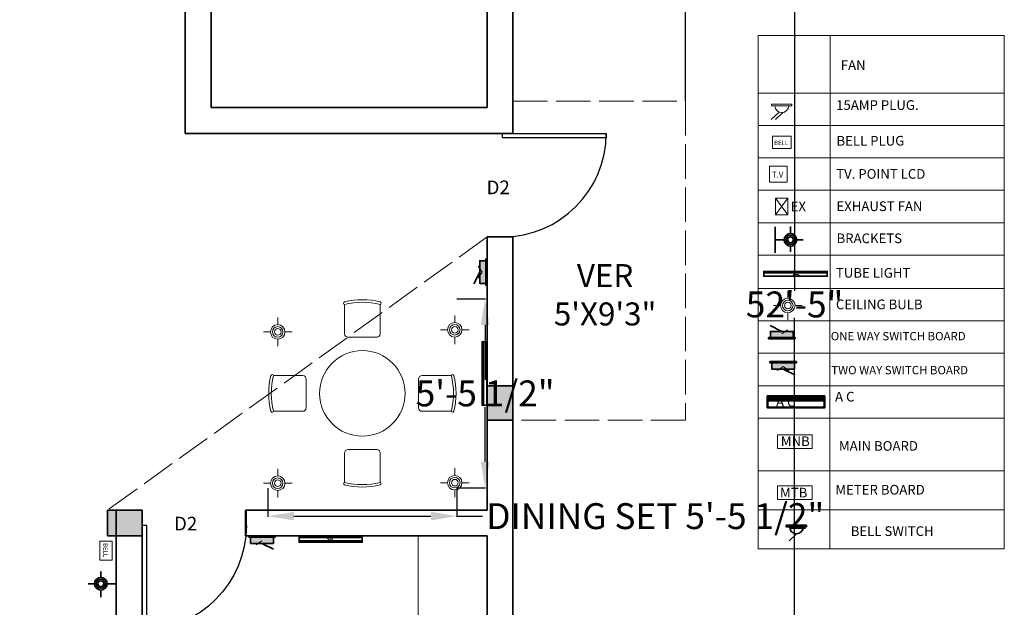
# Model space of a CAD drawing. Units: inches. Extents: x 68 to 1275, y 90 to 1276.
# Tile 5 of 6: x 916 to 1259, y 813 to 1017. Entities that reach past the tile are written whole.
import ezdxf

# ---------------------------------------------------------------- set-up
doc = ezdxf.new("R2010")
doc.units = ezdxf.units.IN
doc.header["$MEASUREMENT"] = 0
doc.linetypes.add('ACAD_ISO02W100', pattern=[15, 12, -3])
for name, color, linetype, lineweight in [('A -Elec', 6, 'Continuous', 18), ('A-ANNO-TEXT', 7, 'Continuous', 18), ('A-AREA-IDEN', 7, 'Continuous', 18), ('A-FLOR-FIXT', 9, 'Continuous', 18), ('A-FLOR-OVHD', 8, 'ACAD_ISO02W100', 13), ('A-WALL', 7, 'Continuous', 35), ('COLUMN', 150, 'Continuous', 35), ('DIM', 2, 'Continuous', 18), ('DOOR', 15, 'Continuous', 25), ('E-ANNO-LEGD', 8, 'Continuous', 13), ('E-ANNO-TEXT', 7, 'Continuous', 18), ('E-EQPM', 1, 'Continuous', 18), ('E-LITE', 6, 'Continuous', 18), ('E-POWR', 1, 'Continuous', 18), ('E-REFR', 8, 'ACAD_ISO02W100', 13), ('Elec', 1, 'Continuous', 35), ('FURN', 163, 'Continuous', 18)]:
    doc.layers.add(name, color=color, linetype=linetype, lineweight=lineweight)
doc.styles.get("Standard").update_dxf_attribs({"font": 'arial.ttf'})
doc.dimstyles.get("Standard").update_dxf_attribs({"dimtxt": 9, "dimasz": 9, "dimexe": 0.18, "dimexo": 0.0625, "dimgap": 0.09, "dimtad": 0, "dimtih": 1, "dimtoh": 1, "dimdec": 1, "dimzin": 0, "dimdsep": 46, "dimlunit": 3, "dimtxsty": 'Standard', "dimcen": 0.09, "dimadec": 0, "dimazin": 0, "dimtfac": 1, "dimtdec": 1, "dimtofl": 0, "dimtmove": 0, "dimatfit": 3, "dimfxl": 1, "dimtolj": 1, "dimtzin": 0, "dimarcsym": 0})

# ---------------------------------------------------------------- blocks, each defined once
blk = doc.blocks.new('*U2')
for p, q in [((0, 0), (-1e-16, -5.999999999999999)), ((40, -6e-16), (40, -6))]:
    blk.add_line(p, q)
blk.add_lwpolyline([(0, 0), (5.6e-15, 40), (1.750000000000007, 40), (1.749999999999998, -7e-16)], close=True)
blk.add_arc((0, 0), 40, 0, 90)
blk = doc.blocks.new('C')
h = blk.add_hatch(color=256)
h.dxf.hatch_style = 1
h.paths.add_polyline_path([(745.8101109123093, 845.9819968167334), (745.8101109123093, 857.9819968167335), (736.8101109123093, 857.9819968167335), (736.8101109123093, 845.9819968167334)])
for p, q in [((745.8101109123093, 857.9819968167335), (736.8101109123093, 857.9819968167335)), ((736.8101109123093, 857.9819968167335), (736.8101109123093, 845.9819968167334)), ((745.8101109123093, 845.9819968167334), (745.8101109123093, 857.9819968167335)), ((736.8101109123093, 845.9819968167334), (745.8101109123093, 845.9819968167334))]:
    blk.add_line(p, q)
blk = doc.blocks.new('DCHARRND')
for p, q in [((-10, -2.638149999995254), (-10, -18.99994999999526)), ((10, -18.99994999999526), (10, -2.638149999995254)), ((-8, -20.99994999999526), (8, -20.99994999999526))]:
    blk.add_line(p, q)
for centre, radius, start, end in [((0, -41.27199999999525), 41.27199999999525, 75.97797000000331, 104.0219999999933), ((-9.769699999999943, -1.946949999995245), 0.7532336000029903, 107.8004999997948, 188.6619999997561), ((-9.86489999999992, -2.000049999995248), 0.6522302000032755, 185.3118999999788, 258.0499999996009), ((0, -42.68031999999524), 41.27199999999525, 75.97797000000331, 104.0219999999933), ((9.769700000000057, -1.946949999995245), 0.7532335999955265, 351.3380000002426, 72.19952999994322), ((9.865000000000009, -2.000049999995248), 0.6522301999967041, 281.9500000003992, 354.6881000000212), ((-8, -18.99994999999526), 2, 180, 270), ((8, -18.99994999999526), 2, 270, 0)]:
    blk.add_arc(centre, radius, start, end)
blk = doc.blocks.new('*U23')
at = {"layer": 'FURN', "xscale": -0.8325683909312864, "yscale": 0.8325683909312864, "zscale": 0.8325683909312864, "rotation": 270}
blk.add_blockref('DCHARRND', (8.741947290566713, 3.1832e-12), dxfattribs=at)
blk = doc.blocks.new('*U24')
at = {"color": 0, "linetype": 'ByBlock', "lineweight": -2, "transparency": 16777216}
for p, rotation in [((1883.427219751119, 1330.162309104793), 90.00000000000006), ((1848.567433110135, 1295.302522463815), 180), ((1883.427219751113, 1260.442735822831), 270.0000000000001)]:
    blk.add_blockref('*U23', p, dxfattribs=dict(at, rotation=rotation))
blk.add_blockref('*U23', (1918.287006392097, 1295.302522463809), dxfattribs=at)
blk = doc.blocks.new('DIN')
blk.add_circle((1883.427219751116, 1295.302522463812), 19.90213577479114)
blk.add_blockref('*U24', (0, 0))
blk = doc.blocks.new('BELL SWITCH')
at = {"layer": 'Elec'}
for p, q in [((4981.810695824261, 3401.308516663301), (4981.810695824261, 3402.267205949833)), ((4981.810695824261, 3402.267205949833), (4993.567325880143, 3402.267205949833)), ((4993.567325880143, 3401.308516663301), (4981.810695824261, 3401.308516663301)), ((4993.567325880143, 3402.267205949833), (4993.567325880143, 3401.308516663301)), ((4987.689010852202, 3397.361748155474), (4983.521874140887, 3393.30038126191))]:
    blk.add_line(p, q, dxfattribs=at)
blk.add_arc((4987.689010852202, 3401.308516663301), 3.946768507828181, 180, 0, dxfattribs=at)
blk = doc.blocks.new('splight')
at = {"layer": 'Elec'}
for p, q in [((4618.165493646445, 527.1595508907546), (4627.57380882646, 527.1595508907546)), ((4622.869651236451, 527.1595508907546), (4622.869651236451, 523.8688723625129)), ((4620.576181531769, 521.5754026578305), (4618.052205676129, 521.5754026578305)), ((4625.163120941137, 521.5754026578305), (4627.232633020232, 521.5754026578305)), ((4622.869651236451, 519.2819329531479), (4622.869651236451, 517.0346704452847))]:
    blk.add_line(p, q, dxfattribs=at)
for radius in [2.293469704682637, 1.668469704682639, 1.043469704682639]:
    blk.add_circle((4622.869651236451, 521.5754026578305), radius, dxfattribs=at)
blk = doc.blocks.new('CIELING')
at = {"layer": 'A -Elec'}
for p, q in [((1070.869500591183, -8395.655580837194), (1070.869500591183, -8391.485789029257)), ((1066.613971407157, -8399.911110021205), (1062.44417959922, -8399.911110021205)), ((1075.125029775208, -8399.911110021205), (1079.294821583145, -8399.911110021205)), ((1070.869500591183, -8408.33643101315), (1070.869500591183, -8404.166639205214))]:
    blk.add_line(p, q, dxfattribs=at)
for radius in [4.255529184009533, 3.095842734009534, 1.936156284009533]:
    blk.add_circle((1070.869500591183, -8399.911110021205), radius, dxfattribs=at)
blk = doc.blocks.new('tube')
at = {"layer": 'A -Elec'}
for p, q in [((4592.607752765609, 556.7543292074987), (4641.607752765609, 556.7543292074987)), ((4592.607752765609, 555.2543292074988), (4592.607752765609, 556.7543292074987)), ((4592.607752765609, 552.7543292074987), (4592.607752765609, 555.2543292074988)), ((4592.607752765609, 552.7543292074987), (4641.607752765609, 552.7543292074987)), ((4593.107752765609, 555.2543292074988), (4593.107752765609, 556.7543292074987)), ((4593.107752765609, 556.3299144522243), (4593.407752765609, 556.3299144522243)), ((4593.107752765609, 556.2104979518087), (4593.407752765609, 556.2104979518087)), ((4593.107752765609, 555.8060867251079), (4593.407752765609, 555.8060867251079)), ((4593.107752765609, 555.6866702246923), (4593.407752765609, 555.6866702246923)), ((4641.107752765608, 555.2543292074988), (4593.107752765609, 555.2543292074988)), ((4593.107752765609, 555.2543292074988), (4593.107752765609, 553.2543292074988)), ((4593.107752765609, 553.2543292074988), (4593.107752765609, 555.2543292074988)), ((4593.107752765609, 553.2543292074988), (4641.607752765609, 553.2543292074988)), ((4593.407752765609, 555.2543292074988), (4593.407752765609, 556.7543292074987)), ((4593.407752765609, 556.5043292074988), (4640.807752765609, 556.5043292074988)), ((4593.407752765609, 556.2543292074987), (4640.807752765609, 556.2543292074987)), ((4593.407752765609, 556.0043292074988), (4640.807752765609, 556.0043292074988)), ((4593.407752765609, 555.7543292074988), (4640.807752765609, 555.7543292074988)), ((4593.407752765609, 555.5043292074988), (4640.807752765609, 555.5043292074988)), ((4640.807752765609, 555.2543292074988), (4640.807752765609, 556.7543292074987)), ((4640.807752765609, 556.3299144522243), (4641.107752765608, 556.3299144522243)), ((4640.807752765609, 556.2104979518087), (4641.107752765608, 556.2104979518087)), ((4640.807752765609, 555.8060867251079), (4641.107752765608, 555.8060867251079)), ((4640.807752765609, 555.6866702246923), (4641.107752765608, 555.6866702246923)), ((4641.107752765608, 556.7543292074987), (4641.107752765608, 555.2543292074988)), ((4641.107752765608, 555.2543292074988), (4641.107752765608, 556.7543292074987)), ((4641.107752765608, 553.2543292074988), (4641.107752765608, 555.2543292074988)), ((4641.607752765609, 556.7543292074987), (4641.607752765609, 555.2543292074988)), ((4641.607752765609, 552.7543292074987), (4641.607752765609, 555.2543292074988))]:
    blk.add_line(p, q, dxfattribs=at)
for points in [[(4615.603450108063, 553.2543292074988), (4619.112055423154, 553.2543292074988), (4619.112055423154, 554.3062122222327), (4615.603450108063, 554.3062122222327)], [(4619.112055423154, 553.7802707148657), (4619.112055423154, 553.7802707148657), (4619.112055423154, 553.7802707148657), (4619.112055423154, 553.7802707148657)], [(4619.112055423154, 553.7802707148657), (4619.813791770798, 553.7802707148657), (4619.813791770798, 553.2543292074988), (4619.112055423154, 553.2543292074988)]]:
    blk.add_lwpolyline(points, close=True, dxfattribs=at)
blk = doc.blocks.new('ac')
at = {"layer": 'Elec'}
for p, q in [((12718.33512872629, -53.78451556294852), (12674.35721837807, -53.78451556294852)), ((12674.35721837806, -63.01930683579224), (12674.35721837807, -53.78451556294852)), ((12674.88506837807, -57.52248662285011), (12717.80727872628, -57.52248662285011)), ((12675.81311487755, -57.52248662285011), (12675.81311487755, -53.78451556294851)), ((12717.02869991749, -54.85019267976269), (12675.81311487755, -54.85019267976269)), ((12717.02869991749, -56.20859049643797), (12675.81311487755, -56.20859049643797)), ((12717.02869991748, -57.52248662285011), (12717.02869991749, -53.78451556294851)), ((12718.33512872629, -63.01930683579224), (12718.33512872629, -53.78451556294852)), ((12718.33512872629, -63.01930683579224), (12674.35721837806, -63.01930683579224))]:
    blk.add_line(p, q, dxfattribs=at)
at = {"layer": 'Elec', "ltscale": 0.1}
for p, q in [((12674.88506837807, -61.49145683579366), (12674.88506837807, -53.78451556294851)), ((12717.02869991749, -54.35872395628861), (12675.81311487755, -54.35872395628861)), ((12717.02869991749, -55.65507023101156), (12675.81311487755, -55.65507023101157)), ((12717.02869991749, -56.84485043173038), (12675.81311487755, -56.84485043173037)), ((12717.80727872628, -61.49145683579366), (12717.80727872628, -53.78451556294851)), ((12716.80727872628, -62.49145683579365), (12675.88506837807, -62.49145683579365))]:
    blk.add_line(p, q, dxfattribs=at)
at = {"layer": 'Elec'}
for centre, start, end in [((12675.88506837807, -61.49145683579366), 180, 270), ((12716.80727872628, -61.49145683579366), 270, 0)]:
    blk.add_arc(centre, 1, start, end, dxfattribs=at)
blk = doc.blocks.new('elec box')
at = {"layer": 'Elec'}
blk.add_hatch(color=256, dxfattribs=at).paths.add_polyline_path([(3828.234962737587, 599.2881263179643), (3828.234962737587, 594.7881263179643), (3844.734962737589, 594.7881263179643), (3844.734962737589, 599.2881263179643)])
for p, q in [((3836.484962737588, 599.2881263179643), (3828.066979685118, 603.4529863194257)), ((3846.10280273742, 594.7881263179643), (3826.830962060027, 594.7881263179643)), ((3826.830962060027, 594.7881263179643), (3826.830962060027, 593.8893551118417)), ((3826.830962060027, 593.8893551118417), (3846.10280273742, 593.8893551118417)), ((3846.10280273742, 593.8893551118417), (3846.10280273742, 594.7881263179643))]:
    blk.add_line(p, q, dxfattribs=at)
blk.add_lwpolyline([(3828.234962737587, 594.7881263179643), (3828.234962737587, 599.2881263179643), (3844.734962737589, 599.2881263179643), (3844.734962737589, 594.7881263179643), (3828.234962737587, 594.7881263179643)], dxfattribs=at)
blk = doc.blocks.new('SWITCHBOARD-ONE-WAY')
blk.add_line((4.634474659967281, 1.72886330620372), (6.643170124125163, 3.124132868275296))
at = {"xscale": 0.480395109260985, "yscale": 0.480395109260985, "zscale": 0.480395109260985}
blk.add_blockref('elec box', (-1838.391242964724, -285.3017071861163), dxfattribs=at)
blk = doc.blocks.new('SWITCHBOARD-TWO-WAY')
for p, q in [((4.623595448308151, 2.865329432813496), (2.614899984150042, 1.47005987070861)), ((4.623595442911664, 2.865329432846692), (6.622900514750199, 1.456637185270096))]:
    blk.add_line(p, q)
at = {"xscale": 0.480395109260985, "yscale": 0.480395109260985, "zscale": 0.480395109260985, "rotation": 180}
blk.add_blockref('elec box', (1847.649313070309, 289.8958999251334), dxfattribs=at)
blk = doc.blocks.new('BELL-POINT')
blk.add_lwpolyline([(1.95874658857e-05, 4.272243527406885), (6.55734876643055, 4.272243527406885), (6.55734876643055, -0.0002228979699339), (1.95874658857e-05, -0.0002228979699339)], close=True)
at = {"insert": (0.6440248614437678, 2.798299889551913), "char_height": 1.537264349632867, "attachment_point": 1}
blk.add_mtext('BELL', dxfattribs=at)
blk = doc.blocks.new('TV-POINT')
blk.add_lwpolyline([(2.2128117507e-06, 5.568118865895371), (6.100736396045249, 5.568118865895371), (6.100736396045249, -7.01044664311e-05), (2.2128117507e-06, -7.01044664311e-05)], close=True)
at = {"transparency": 33554676}
blk.add_lwpolyline([(2.2128117507e-06, 5.568118865895371), (6.100736396045249, 5.568118865895371), (6.100736396045249, -7.01044664311e-05), (2.2128117507e-06, -7.01044664311e-05)], close=True, dxfattribs=at)
at = {"insert": (0.8393167226115565, 3.647168321161302), "char_height": 2.003474701485161, "attachment_point": 1}
blk.add_mtext('T.V ', dxfattribs=at)
at = {"transparency": 33554676, "insert": (0.8393167226115565, 3.647168321161302), "char_height": 2.003474701485161, "attachment_point": 1}
blk.add_mtext('T.V ', dxfattribs=at)
blk = doc.blocks.new('MAIN-BOARD')
blk.add_lwpolyline([(0.0004361200251424, 4.703133274055858), (12.06279134155943, 4.703133274055858), (12.06279134155943, 0.0003298403245253), (0.0004361200251424, 0.0003298403245253)], close=True)
blk.add_text('MNB', height=3.362765764821897).set_placement((1.14402048200327, 0.7969751531460361))
blk = doc.blocks.new('METER-BOARD')
blk.add_lwpolyline([(0.0004361200251424, 4.702354804303354), (12.06279134155943, 4.702354804303354), (12.06279134155943, -0.0004486294279786), (0.0004361200251424, -0.0004486294279786)], close=True)
blk.add_text('MTB', height=3.362765764821897).set_placement((0.8731259797250459, 0.6934873088445102))
blk = doc.blocks.new('*D65')
at = {"layer": 'Defpoints', "color": 0, "transparency": 16777216}
for p in [(1002.392096138563, 854.1861430656332), (1068.072978243499, 854.1861430656332), (1068.072978243499, 844.3340107498929)]:
    blk.add_point(p, dxfattribs=at)
at = {"layer": 'DIM', "color": 0, "lineweight": -2, "transparency": 16777216}
for p, q in [((1002.392096138563, 854.1236430656332), (1002.392096138563, 844.1540107498928)), ((1068.072978243499, 854.1236430656332), (1068.072978243499, 844.1540107498928)), ((1011.392096138563, 844.3340107498929), (1059.072978243499, 844.3340107498929)), ((1068.072978243499, 844.3340107498929), (1077.072978243499, 844.3340107498929))]:
    blk.add_line(p, q, dxfattribs=at)
at = {"layer": 'DIM', "color": 0, "transparency": 16777216}
for points in [[(1011.392096138563, 845.8340107498926), (1011.392096138563, 842.8340107498927), (1002.392096138563, 844.3340107498929)], [(1059.072978243499, 845.8340107498926), (1059.072978243499, 842.8340107498927), (1068.072978243499, 844.3340107498929)]]:
    blk.add_solid(points, dxfattribs=at)
at = {"layer": 'DIM', "color": 0, "transparency": 16777216, "insert": (1137.108749048411, 844.3340107498929), "char_height": 9, "attachment_point": 5}
blk.add_mtext('\\A1;DINING SET 5\'-5 1/2"', dxfattribs=at)
blk = doc.blocks.new('*D66')
at = {"layer": 'Defpoints', "color": 0, "transparency": 16777216}
for p in [(1068.0729782435, 919.8670251705701), (1077.92511055924, 919.8670251705701), (1068.0729782435, 854.1861430656338)]:
    blk.add_point(p, dxfattribs=at)
at = {"layer": 'DIM', "color": 0, "lineweight": -2, "transparency": 16777216}
for p, q in [((1068.1354782435, 919.8670251705701), (1078.10511055924, 919.8670251705701)), ((1077.92511055924, 910.8670251705701), (1077.92511055924, 891.7700629721265)), ((1077.92511055924, 863.1861430656337), (1077.92511055924, 882.2831052640774)), ((1068.1354782435, 854.1861430656338), (1078.10511055924, 854.1861430656338))]:
    blk.add_line(p, q, dxfattribs=at)
at = {"layer": 'DIM', "color": 0, "transparency": 16777216}
for points in [[(1076.425110559241, 910.8670251705701), (1079.42511055924, 910.8670251705701), (1077.92511055924, 919.8670251705701)], [(1076.425110559241, 863.1861430656337), (1079.42511055924, 863.1861430656337), (1077.92511055924, 854.1861430656338)]]:
    blk.add_solid(points, dxfattribs=at)
at = {"layer": 'DIM', "color": 0, "transparency": 16777216, "insert": (1077.92511055924, 887.0265841181014), "char_height": 9, "attachment_point": 5}
blk.add_mtext('\\A1;5\'-5 1/2"', dxfattribs=at)
blk = doc.blocks.new('*D112')
at = {"layer": 'Defpoints', "color": 0, "transparency": 16777216}
for p in [(1147.626284, 1270.418609), (718.626284, 1232.468609), (1147.626284, 988.6789849999999)]:
    blk.add_point(p, dxfattribs=at)
at = {"layer": 'DIM', "color": 0, "lineweight": -2, "transparency": 16777216}
for p, q in [((718.626284, 1232.531109), (718.626284, 1270.598609)), ((727.626284, 1270.418609), (917.5809633997271, 1270.418609)), ((1138.626284, 1270.418609), (948.6716046002728, 1270.418609)), ((1147.626284, 988.741485), (1147.626284, 1270.598609))]:
    blk.add_line(p, q, dxfattribs=at)
at = {"layer": 'DIM', "color": 0, "transparency": 16777216}
for points in [[(727.626284, 1271.918609), (727.626284, 1268.918609), (718.626284, 1270.418609)], [(1138.626284, 1271.918609), (1138.626284, 1268.918609), (1147.626284, 1270.418609)]]:
    blk.add_solid(points, dxfattribs=at)
at = {"layer": 'DIM', "color": 0, "transparency": 16777216, "insert": (933.1262839999999, 1270.418609), "char_height": 9, "attachment_point": 5}
blk.add_mtext('\\A1;35\'-9"', dxfattribs=at)
blk = doc.blocks.new('*D113')
at = {"layer": 'Defpoints', "color": 0, "transparency": 16777216}
for p in [(1087.626284, 1232.468609), (1185.576284000001, 1232.468609), (1087.626284, 603.4686090000002)]:
    blk.add_point(p, dxfattribs=at)
at = {"layer": 'DIM', "color": 0, "lineweight": -2, "transparency": 16777216}
for p, q in [((1087.688784, 1232.468609), (1185.756284000001, 1232.468609)), ((1185.576284000001, 1223.468609), (1185.576284000001, 922.6537658894956)), ((1185.576284000001, 612.4686090000002), (1185.576284000001, 913.2834521105051)), ((1087.688784, 603.4686090000002), (1185.756284000001, 603.4686090000002))]:
    blk.add_line(p, q, dxfattribs=at)
at = {"layer": 'DIM', "color": 0, "transparency": 16777216}
for points in [[(1184.076284000001, 1223.468609), (1187.076284000001, 1223.468609), (1185.576284000001, 1232.468609)], [(1184.076284000001, 612.4686090000002), (1187.076284000001, 612.4686090000002), (1185.576284000001, 603.4686090000002)]]:
    blk.add_solid(points, dxfattribs=at)
at = {"layer": 'DIM', "color": 0, "transparency": 16777216, "insert": (1185.576284000001, 917.9686089999998), "char_height": 9, "attachment_point": 5}
blk.add_mtext('\\A1;52\'-5"', dxfattribs=at)

msp = doc.modelspace()

# ---------------------------------------------------------------- linework, layer by layer
at = {"layer": 'A-FLOR-FIXT'}
msp.add_line((1054.626283693841, 837.4686089321809), (1054.626283693841, 729.4686089321808), dxfattribs=at)
at = {"layer": 'A-FLOR-OVHD'}
for p, q in [((1087.626283693841, 988.6789849601155), (1147.626283693841, 988.6789849601155)), ((1147.626283693841, 988.6789849601155), (1147.626283693841, 877.6789849601154)), ((1147.626283693841, 877.6789849601154), (1087.626283693841, 877.6789849601154))]:
    msp.add_line(p, q, dxfattribs=at)
at = {"layer": 'A-WALL'}
for p, q in [((1087.626283693841, 1232.468608932181), (1087.626283693841, 977.4686089321807)), ((973.626283693841, 1082.468608932181), (973.626283693841, 977.4686089321807)), ((982.626283693841, 1082.468608932181), (982.626283693841, 986.4686089321807)), ((1078.626283693841, 1082.468608932181), (1078.626283693841, 986.4686089321807)), ((982.626283693841, 986.4686089321807), (1078.626283693841, 986.4686089321807)), ((973.626283693841, 977.4686089321807), (1078.626283693841, 977.4686089321807)), ((1078.626283693841, 977.4686089321807), (1087.626283693841, 977.4686089321807)), ((1078.626283693841, 941.4686089321808), (1078.626283693841, 846.4686089321808)), ((1078.626283693841, 941.4686089321808), (1087.626283693841, 941.4686089321808)), ((1087.626283693841, 941.4686089321808), (1087.626283693841, 696.4686089321808)), ((949.6262836938411, 846.4686089321808), (958.6262836938411, 846.4686089321808)), ((949.6262836938411, 846.4686089321808), (949.6262836938411, 705.4686089321807)), ((958.6262836938411, 837.4686089321809), (958.6262836938411, 846.4686089321808)), ((994.626283693841, 846.4686089321808), (1078.626283693841, 846.4686089321808)), ((994.626283693841, 837.4686089321809), (994.626283693841, 846.4686089321808)), ((949.6262836938411, 837.4686089321809), (958.6262836938411, 837.4686089321809)), ((958.6262836938411, 837.4686089321809), (958.6262836938411, 705.4686089321807)), ((994.626283693841, 837.4686089321809), (1078.626283693841, 837.4686089321809)), ((1078.626283693841, 837.4686089321809), (1078.626283693841, 705.4686089321807))]:
    msp.add_line(p, q, dxfattribs=at)
at = {"layer": 'E-ANNO-LEGD'}
for p, q in [((1172.946309647792, 832.969593099326), (1172.946309647792, 1011.519571694431)), ((1258.530314853673, 1011.519571694431), (1172.946309647792, 1011.519571694431)), ((1197.924334482565, 1011.519571694431), (1197.781428473779, 832.969593099326)), ((1258.530314853665, 832.969593099326), (1258.530314853665, 1011.519571694431)), ((1258.530314853673, 991.4346260608072), (1172.946309647792, 991.4346260608072)), ((1258.530314853673, 991.4346260608239), (1172.946309647792, 991.4346260608239)), ((1258.530314853673, 980.1762997075286), (1172.946309647792, 980.1762997075286)), ((1258.530314853665, 968.9179733542502), (1172.946309647775, 968.9179733542502)), ((1258.530314853673, 957.6596470009549), (1172.946309647792, 957.6596470009549)), ((1258.530314853673, 946.4013206476765), (1172.946309647792, 946.4013206476765)), ((1258.530314853673, 935.142994294398), (1172.946309647792, 935.142994294398)), ((1258.530314853665, 923.4772036206607), (1172.946309647775, 923.4772036206607)), ((1258.530314853665, 912.2188772673657), (1172.946309647775, 912.2188772673657)), ((1258.530314853665, 900.960550914087), (1172.946309647775, 900.960550914087)), ((1258.530314853673, 889.702224560792), (1172.946309647792, 889.702224560792)), ((1258.530314853673, 878.4438982075135), (1172.946309647792, 878.4438982075135)), ((1258.530314853673, 860.0415084382558), (1172.946309647792, 860.0415084382558)), ((1258.530314853673, 846.505550768799), (1172.946309647792, 846.505550768799)), ((1258.530314853673, 832.9695930993256), (1172.946309647792, 832.9695930993256))]:
    msp.add_line(p, q, dxfattribs=at)
at = {"layer": 'E-EQPM'}
for p, q in [((1178.958906185277, 954.9375739626636), (1183.282462168619, 949.1728326515301)), ((1183.282462168619, 954.9375739626636), (1178.958906185277, 949.1728326515301))]:
    msp.add_line(p, q, dxfattribs=at)
msp.add_lwpolyline([(1183.282462168619, 954.9375739626636), (1178.958906185277, 954.9375739626636), (1178.958906185277, 949.1728326515301), (1183.282462168619, 949.1728326515301)], close=True, dxfattribs=at)
at = {"layer": 'E-POWR'}
for p, q in [((1177.590791939301, 987.6368285849791), (1184.650576414587, 987.6368285849791)), ((1177.590791939301, 987.06114152929), (1177.590791939301, 987.6368285849791)), ((1184.650576414587, 987.06114152929), (1177.590791939301, 987.06114152929)), ((1184.650576414587, 987.6368285849791), (1184.650576414587, 987.06114152929)), ((1180.178658963754, 984.8863915189612), (1177.475973345754, 982.2523051778636)), ((1181.47769277534, 984.6911311686061), (1178.975352655661, 982.2523051778636))]:
    msp.add_line(p, q, dxfattribs=at)
msp.add_arc((1181.120684176957, 987.06114152929), 2.370010360678894, 180, 0, dxfattribs=at)
at = {"layer": 'E-REFR'}
msp.add_line((1078.626283693841, 941.4425014682521), (946.626283693841, 846.4686089321808), dxfattribs=at)

# ---------------------------------------------------------------- block references
at = {"layer": 'COLUMN'}
msp.add_blockref('C', (341.8161727815318, 31.69698814338199), dxfattribs=at)
at = {"layer": 'COLUMN', "rotation": 270}
msp.add_blockref('C', (100.6442868771076, 1583.27871984449), dxfattribs=at)
at = {"layer": 'DOOR'}
for p, xscale, yscale, zscale, rotation in [((1084.03019981343, 977.4686089321807), 0.9006526865982184, 0.9006526865982184, 0.9006526865982184, 270), ((958.6262836938411, 841.0323348320559), -0.9060456833541303, 0.9060456833541303, 0.9060456833541303, 180)]:
    msp.add_blockref('*U2', p, dxfattribs=dict(at, xscale=xscale, yscale=yscale, zscale=zscale, rotation=rotation))
at = {"layer": 'E-EQPM', "xscale": 0.4550488862921059, "yscale": 0.4550488862921059, "zscale": 0.4550488862921059}
msp.add_blockref('ac', (-4591.407624430582, 910.6272418164888), dxfattribs=at)
at = {"layer": 'E-LITE', "xscale": -0.9617510087435096, "yscale": 0.9617510087435096, "zscale": 0.9617510087390623}
for p, rotation in [((1685.776876615766, 5386.48438017791), 89.99999999999976), ((442.6300538558616, -3625.202949076657), 269.9999999999998)]:
    msp.add_blockref('splight', p, dxfattribs=dict(at, rotation=rotation))
at = {"layer": 'E-LITE', "transparency": 33554676}
for name, p, xscale, yscale, zscale in [('tube', (-907.8172856470304, 677.0348467610315), 0.4534687213066354, 0.4534687213066354, 0.4534687213066354), ('CIELING', (548.1277733358314, 5899.191783018319), 0.5930528030907906, 0.5930528030907906, 0.5930528030907906), ('CIELING', (370.6979267614556, 5890.015012933644), 0.5930528030907906, 0.5930528030907906, 0.5930528030907906), ('CIELING', (432.2742816529547, 5890.740989383461), 0.5930528030907906, 0.5930528030907906, 0.5930528030907906), ('CIELING', (370.6979267614555, 5837.381712511994), 0.5930528030907906, 0.5930528030907906, 0.5930528030907906), ('CIELING', (432.2742816529547, 5837.56320705833), 0.5930528030907906, 0.5930528030907906, 0.5930528030907906)]:
    msp.add_blockref(name, p, dxfattribs=dict(at, xscale=xscale, yscale=yscale, zscale=zscale))
at = {"layer": 'E-LITE', "transparency": 33554676, "xscale": 0.4534687213066354, "yscale": 0.4534687213066354, "zscale": 0.4534687213066354}
for p, rotation in [((1329.283082556272, -1199.745339849393), 90), ((3117.919190103777, 1087.649408450732), 180)]:
    msp.add_blockref('tube', p, dxfattribs=dict(at, rotation=rotation))
at = {"layer": 'E-POWR'}
for name, p in [('BELL-POINT', (1177.842, 972.16)), ('TV-POINT', (1176.86, 960.4409999999999)), ('SWITCHBOARD-ONE-WAY', (1176.492, 906.0109999999999)), ('SWITCHBOARD-TWO-WAY', (1176.956, 893.468)), ('MAIN-BOARD', (1179.649, 867.9149999999998)), ('METER-BOARD', (1179.649, 850.131))]:
    msp.add_blockref(name, p, dxfattribs=at)
for name, p, rotation in [('SWITCHBOARD-TWO-WAY', (1074.031925406596, 933.8392687714955), 269.9999999999983), ('SWITCHBOARD-ONE-WAY', (1004.945216716659, 837.4684433839535), 180), ('BELL-POINT', (943.8853808516823, 835.6273728276122), 270.0000000000045)]:
    msp.add_blockref(name, p, dxfattribs=dict(at, rotation=rotation))
at = {"layer": 'E-POWR', "xscale": 0.6004938865802444, "yscale": 0.6004938865802444, "zscale": 0.6004938865802444}
msp.add_blockref('BELL SWITCH', (-1808.840048966689, -1201.889676666774), dxfattribs=at)
at = {"layer": 'FURN', "xscale": 0.7473412872623325, "yscale": 0.7473412872623325, "zscale": 0.7473412872623325}
msp.add_blockref('DIN', (-372.330385682684, -81.00647041415014), dxfattribs=at)

# ---------------------------------------------------------------- texts
at = {"layer": 'A-ANNO-TEXT', "char_height": 5.953076141217599, "width": 20.39887023007676, "attachment_point": 5}
for insert in [(1082.485696791979, 958.6761441380895), (973.7493967042031, 841.7440509360767)]:
    msp.add_mtext('{\\fTimes New Roman|b0|i0|c0|p18;\\H0.8x;D2}', dxfattribs=dict(at, insert=insert))
at = {"layer": 'A-AREA-IDEN', "insert": (1119.672051694702, 931.9957913969266), "char_height": 8, "attachment_point": 2}
msp.add_mtext_dynamic_manual_height_columns('VER\\P5\'X9\'3"', width=128.8568059801491, gutter_width=1, heights=[0], dxfattribs=at)
at = {"layer": 'E-ANNO-TEXT'}
for s, height, p in [('FAN', 3.362765764821897, (1201.648005831151, 999.4990843051665)), ('15AMP PLUG.', 3.362765764821897, (1200.039740619537, 985.6261593966105)), ('BELL PLUG', 3.362765764821897, (1200.146922723242, 973.2147637125493)), ('TV. POINT LCD', 3.362765764821897, (1200.052939275629, 961.6750603480117)), ('EXHAUST FAN', 3.362765764821897, (1200.14669731923, 950.4371756304228)), ('BRACKETS', 3.362765764821897, (1200.162971487606, 939.2807612537383)), ('TUBE LIGHT', 3.362765764821897, (1199.958655289399, 927.267052449395)), ('CEILING BULB', 3.362765764821897, (1199.95473826888, 916.3046464856975)), ('ONE WAY SWITCH BOARD', 2.913500258641691, (1198.160958747007, 905.4720905206309)), ('TWO WAY SWITCH BOARD', 2.913500258641691, (1198.325316063464, 893.6613318313408)), (' A C', 3.362765764821897, (1198.63307232581, 884.2074911431405)), ('MAIN BOARD', 3.362765764821897, (1201.01314826475, 867.0748685942385)), ('METER BOARD', 3.362765764821897, (1199.764892476477, 851.8481165299453)), ('BELL SWITCH', 3.362765764821897, (1205.106062546468, 837.440294755018))]:
    msp.add_text(s, height=height, dxfattribs=at).set_placement(p)
at = {"layer": 'E-EQPM'}
msp.add_text(' A C', height=3.362765764821897, dxfattribs=at).set_placement((1178.104896180244, 882.4186415535379))
at = {"layer": 'E-EQPM', "insert": (1184.207779912965, 953.7246227418229), "char_height": 3.362765764821897, "width": 5.871009998848781, "attachment_point": 1}
msp.add_mtext('EX', dxfattribs=at)

# ---------------------------------------------------------------- dimensions: what is measured, and where the dimension line sits
at = {"layer": 'DIM'}
dim = msp.add_linear_dim(base=(1147.626284, 1270.418609), p1=(718.626284, 1232.468609), p2=(1147.626284, 988.6789849999999), dimstyle='Standard', override={"dimdec": 1, "dimlfac": 1, "dimrnd": 0, "dimzin": 1, "dimdsep": 46, "dimlunit": 4, "dimfrac": 2}, dxfattribs=at)
dim.commit()
dim.dimension.update_dxf_attribs({"geometry": '*D112', "text_midpoint": (933.1262839999999, 1270.418609)})
for base, p1, p2, picture, middle in [((1185.576284000001, 1232.468609), (1087.626284, 603.468609), (1087.626284, 1232.468609), '*D113', (1185.576284000001, 917.9686089999998)), ((1077.92511055924, 919.8670251705701), (1068.072978243499, 854.1861430656332), (1068.072978243499, 919.8670251705696), '*D66', (1077.92511055924, 887.0265841181014))]:
    dim = msp.add_linear_dim(base=base, p1=p1, p2=p2, angle=90, dimstyle='Standard', override={"dimdec": 1, "dimlfac": 1, "dimrnd": 0, "dimzin": 1, "dimdsep": 46, "dimlunit": 4, "dimfrac": 2}, dxfattribs=at)
    dim.commit()
    dim.dimension.update_dxf_attribs({"geometry": picture, "text_midpoint": middle})
dim = msp.add_linear_dim(base=(1068.072978243499, 844.3340107498929), p1=(1002.392096138563, 854.1861430656332), p2=(1068.072978243499, 854.1861430656332), text='DINING SET <>', dimstyle='Standard', override={"dimdec": 1, "dimlfac": 1, "dimrnd": 0, "dimzin": 1, "dimdsep": 46, "dimlunit": 4, "dimfrac": 2}, dxfattribs=at)
dim.commit()
dim.dimension.update_dxf_attribs({"geometry": '*D65', "text_midpoint": (1137.108749048411, 844.3340107498929)})

doc.saveas('drawing.dxf')
